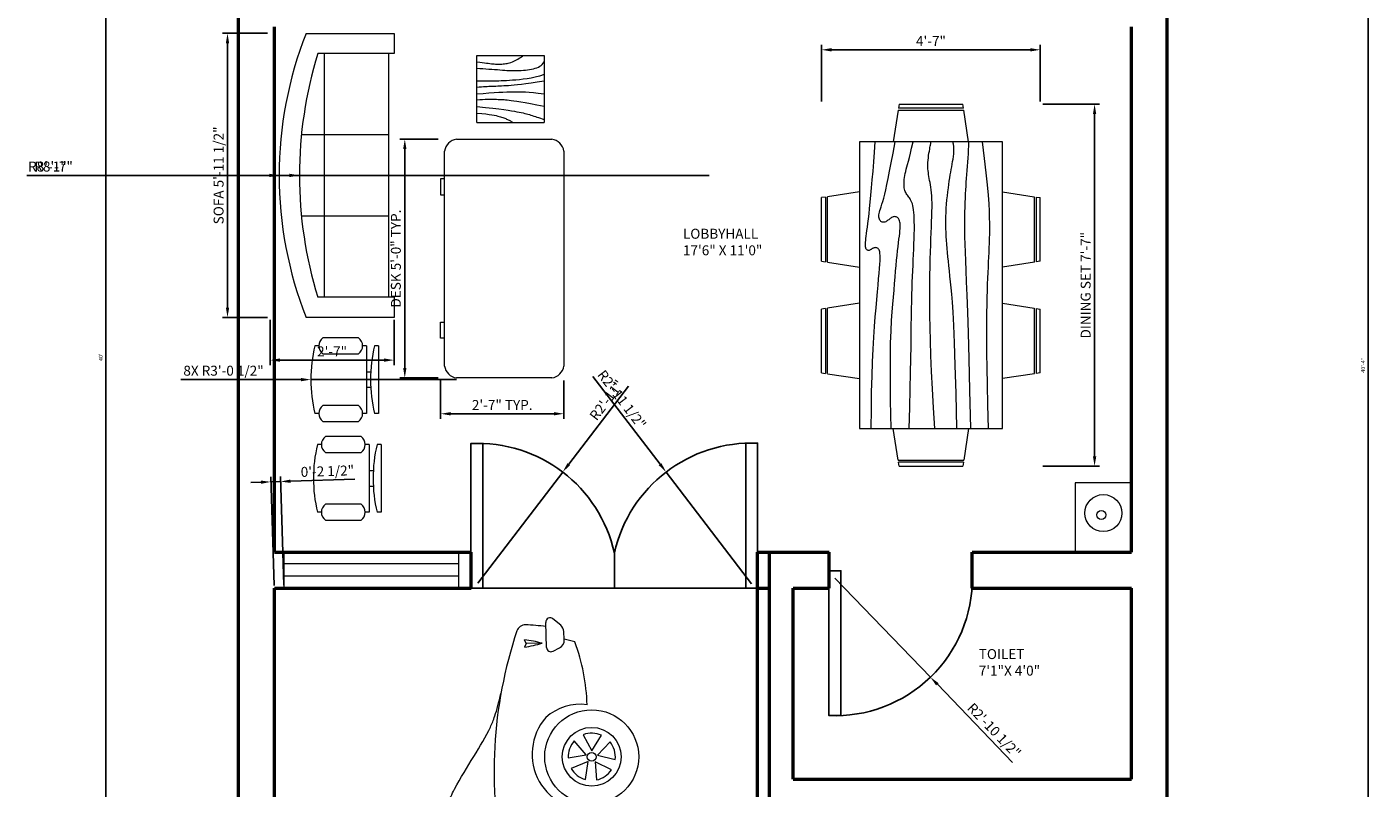
# Model space of a CAD drawing. Units: inches. Extents: x 210 to 950, y 0 to 561.
# Tile 2 of 5: x 210 to 548, y 190 to 382. Entities that reach past the tile are written whole.
import ezdxf

# ---------------------------------------------------------------- set-up
doc = ezdxf.new("R2010")
doc.units = ezdxf.units.IN
for name, color, linetype, lineweight in [('A-ANNO-DIMS', 2, 'Continuous', 18), ('A-AREA-IDEN', 7, 'Continuous', 18), ('A-DOOR', 4, 'Continuous', 25), ('A-FLOR-FIXT', 9, 'Continuous', 18), ('A-FURN', 8, 'Continuous', 18), ('A-GLAZ', 4, 'Continuous', 20), ('A-SITE-VEHI', 8, 'Continuous', 13), ('A-WALL', 7, 'Continuous', 50)]:
    doc.layers.add(name, color=color, linetype=linetype, lineweight=lineweight)
doc.styles.get("Standard").update_dxf_attribs({"font": 'arial.ttf'})
doc.dimstyles.new('ISO-25', dxfattribs={"dimtxt": 2.5, "dimasz": 2.5, "dimexe": 1.25, "dimexo": 0.625, "dimtad": 1, "dimtxsty": 'Standard', "dimcen": 2.5, "dimadec": 0, "dimazin": 0, "dimtfac": 1, "dimtmove": 0, "dimatfit": 3, "dimfxl": 1, "dimarcsym": 0})

# ---------------------------------------------------------------- blocks, each defined once
blk = doc.blocks.new('*U2')
for p, q in [((72.93, 40.23), (85.8, 53.18)), ((75, 38.82), (88.08, 51.97)), ((119.39, 51.91), (117.92, 38.32)), ((50.13, 41.06), (34.31, 40.98)), ((43.26, 39.85), (35.15, 39.78)), ((35.3, 40.46), (50.13, 40.62)), ((111.09, 34.73), (118.48, 34.64)), ((46.65, 26.83), (136.29, 26.77)), ((179.3, 24.35), (180.25, 22.49)), ((180.37, 26.17), (187.51, 26.41)), ((186.68, 22.17), (188.51, 24.37)), ((7.45, 19.78), (9.74, 19.8)), ((10.37, 19.19), (10.38, 18.56)), ((182.62, 21.14), (184.91, 21.28)), ((9.76, 17.93), (8.53, 17.92)), ((50.87, 13.52), (50.91, 10.52))]:
    blk.add_line(p, q)
for points in [[(35.31, 39.93), (35.3, 40.27, 0.269532), (35.14, 40.54), (34.38, 40.96, 0.575383), (34.15, 40.83), (34.15, 40.49, 0.269532), (34.32, 40.22), (35.08, 39.79, 0.575383)], [(28.49, 15.1), (33.61, 14.4), (31.65, 19.18, 0.199906)], [(34.64, 20.05), (35.56, 14.97), (39.5, 18.31, 0.199906)], [(142.85, 15.1), (147.96, 14.4), (146.01, 19.18, 0.199906)], [(148.99, 20.05), (149.91, 14.97), (153.85, 18.31, 0.199906)], [(41.25, 15.74), (36.7, 13.3), (41.09, 10.58, 0.199906)], [(155.6, 15.74), (151.06, 13.3), (155.45, 10.58, 0.199906)], [(31.31, 7.72), (33.55, 12.37), (28.4, 11.99, 0.199906)], [(39.19, 8.12), (35.46, 11.69), (34.23, 6.67, 0.199906)], [(145.66, 7.72), (147.9, 12.37), (142.75, 11.99, 0.199906)], [(153.54, 8.12), (149.81, 11.69), (148.59, 6.67, 0.199906)]]:
    blk.add_lwpolyline(points, format="xyb", close=True)
for points in [[(181.58, 27.46), (181.53, 31.95), (180.48, 32.43)], [(181.58, 27.46), (181.53, 31.95), (182.57, 32.45)], [(50.91, 10.52), (134.38, 11.83)]]:
    blk.add_lwpolyline(points)
for centre, radius in [((115.89, 31.01), 0.619), ((34.98, 13.35), 13.35), ((149.33, 13.35), 13.35), ((34.98, 13.35), 8.35), ((149.33, 13.35), 8.35), ((34.98, 13.35), 1.25), ((149.33, 13.35), 1.25)]:
    blk.add_circle(centre, radius)
for centre, radius, start, end in [((114.6, 105.09), 59.37, 237.6103, 240.9785), ((103.45, -95), 147.78, 83.8163, 95.9705), ((95.51, 3.91), 53.61, 43.2748, 63.5665), ((73.29, 50.49), 10.26, 230.424, 268.0085), ((42.18, -111.35), 149.91, 87.8393, 105.8096), ((20.53, -3.15), 43.06, 98.5304, 116.112), ((80.1, -1364.13), 1402.96, 88.42296, 91.3179), ((118.31, 22.51), 51.16, 161.4307, 193.2363), ((145.17, -84.88), 125.99, 71.5283, 102.1242), ((25.66, 24.94), 94.01, 351.8279, 8.1674), ((184.3, 32.25), 2.49, 357.932, 71.5283), ((79.16, 30.11), 76.3, 177.5773, 185.5205), ((45.64, 26.83), 78.76, 0.852, 4.6556), ((47.43, 26.85), 78.76, 0.852, 4.6556), ((49.23, 26.87), 78.76, 0.852, 4.6556), ((216.26, 37.76), 36.17, 188.4683, 196.5315), ((146.68, 36.98), 36.17, 344.7432, 352.8063), ((116.55, 34.7), 70.29, 353.1942, 357.932), ((34.98, 13.35), 15.9, 0.6373, 176.3412), ((150.1, 14.36), 15.92, 49.2263, 189.1528), ((45.64, 26.83), 78.76, 355.2644, 358.8633), ((47.43, 26.85), 78.76, 355.2644, 358.8633), ((49.23, 26.87), 78.76, 355.2644, 358.8633), ((149.4, 16.55), 14.84, 352.7285, 41.6613), ((180.41, 24.92), 1.25, 91.939, 207.109), ((187.55, 25.16), 1.25, 320.1683, 91.939), ((9.75, 19.18), 0.623, 0.6373, 90.6373), ((182.47, 23.63), 2.49, 207.109, 273.4677), ((114.25, 37.03), 70.29, 344.3985, 346.9385), ((184.76, 23.76), 2.49, 273.4677, 320.1683), ((9.76, 18.55), 0.623, 270.6373, 0.6373), ((162.47, 70.82), 56.18, 271.6865, 290.2774)]:
    blk.add_arc(centre, radius, start, end)
blk.add_ellipse((116.89, 33.59), major_axis=(-0.63, -0.007), ratio=0.610043)
for points, knots in [([(11.39, 38.92), (18.06, 40.19), (30.91, 42.01), (64.77, 40.11), (70.25, 44.91), (82.35, 56.38), (99.18, 57.3), (116.06, 56.35), (133.04, 55.87), (145.24, 49.87), (153.62, 43.8), (161.17, 40.68), (164.92, 39.73), (167.29, 39.15)], [18.629823, 18.629823, 18.629823, 18.629823, 19.527405, 20.700571, 21.107983, 21.608568, 21.92336, 23.151359, 23.716171, 23.908743, 24.77794, 24.943072, 25.187755, 25.187755, 25.187755, 25.187755]), ([(19.11, 14.36), (18.99, 14.21), (18.5, 13.81), (15.35, 15), (9.19, 13.94), (7.26, 22.22), (3.01, 22.66), (1.32, 23.61), (0.64, 26.92), (-0.96, 31.49), (1.54, 32.64), (1.5, 34.06), (1.49, 34.8), (1.49, 35.06), (1.52, 35.3), (1.58, 35.51)], [16.815853, 16.815853, 16.815853, 16.815853, 16.838212, 16.885395, 17.18439, 17.479846, 17.654423, 17.670693, 17.696923, 18.016358, 18.052739, 18.140805, 18.140805, 18.140805, 18.172382, 18.172382, 18.172382, 18.172382])]:
    blk.add_open_spline(points, degree=3, knots=knots)
blk = doc.blocks.new('Sofa - Roundback 7 ft.')
for p, q in [((-12.00002, -32.4421), (-12.00003, -6.5971)), ((11.99997, -32.4421), (11.99998, -6.5971)), ((-36.000027, -34), (-36.000027, -11.4696)), ((35.99998, -34), (35.99998, -11.4696)), ((-35.999844, -13.3819), (35.9998, -13.3819)), ((-36.000027, -32.4421), (35.99998, -32.4421))]:
    blk.add_line(p, q)
for points in [[(-36.000027, -34), (-42.000027, -34), (-42.000027, -8)], [(41.99998, -8), (41.99998, -34), (35.99998, -34)]]:
    blk.add_lwpolyline(points)
for centre, radius, start, end in [((0, -114.25), 114.25, 68.43141, 111.5686), ((-0.00001, -127.1968), 121.1968, 72.72033, 107.2797)]:
    blk.add_arc(centre, radius, start, end)
blk = doc.blocks.new('Chair - Desk')
for p, q in [((-8.5, 0), (-8.5, -1)), ((-8.5, 0), (8.5, 0)), ((8.5, 0), (8.5, -1)), ((-8.5, -3), (-8.5, -4)), ((-8.5, -3), (8.5, -3)), ((-2, -3), (-2, -1.9355)), ((2, -1.9576), (2, -3)), ((8.5, -3), (8.5, -4)), ((-10.5, -5), (-10.5, -14)), ((-6.5, -14), (-6.5, -5)), ((6.5, -5), (6.5, -14)), ((10.5, -14), (10.5, -5)), ((-8.5, -15), (-8.5, -16)), ((8.5, -15), (8.5, -16))]:
    blk.add_line(p, q)
for centre, radius, start, end in [((0, 34.625), 36.625, 256.5803, 283.4197), ((-8.5, -6.5), 2.5, 36.8699, 143.1301), ((8.5, -6.5), 2.5, 36.8699, 143.1301), ((-8.5, -12.5), 2.5, 216.8699, 323.1301), ((0, 19.625), 36.625, 256.5803, 283.4197), ((8.5, -12.5), 2.5, 216.8699, 323.1301)]:
    blk.add_arc(centre, radius, start, end)
blk = doc.blocks.new('Dining Set - 36 x 72 in.')
for p, q in [((-22, 27.5), (-22.1562, 26.50042)), ((-22, 27.5), (-6, 27.5)), ((-5.8437, 26.49966), (-6, 27.5)), ((6, 27.5), (5.8438, 26.50042)), ((6, 27.5), (22, 27.5)), ((22.1563, 26.49966), (22, 27.5)), ((-22.2343, 26.00059), (-23.4847, 17.99762)), ((-22.2304, 26), (-5.7608, 26)), ((-5.8416, 26.5), (-22.1534, 26.5)), ((-4.5152, 17.99762), (-5.7655, 25.99926)), ((5.7657, 26.00059), (4.5153, 17.99762)), ((5.7696, 26), (22.2392, 26)), ((22.1584, 26.5), (5.8466, 26.5)), ((23.4848, 17.99762), (22.2345, 25.99926)), ((36, 18), (-36, 18)), ((-36, 18), (-36, -18)), ((36, -18), (36, 18)), ((-45.5, 8), (-44.5004, 8.15617)), ((-45.5, 8), (-45.5, -8)), ((-44.5, -8.15843), (-44.5, 8.15338)), ((-44.0006, 8.23428), (-35.9976, 9.48474)), ((-44, 8.23041), (-44, -8.23915)), ((44.0006, 8.23428), (35.9976, 9.48474)), ((44, 8.23041), (44, -8.23915)), ((44.5, -8.15843), (44.5, 8.15338)), ((45.5, 8), (44.5005, 8.15617)), ((45.5, 8), (45.5, -8)), ((-44.4997, -8.15631), (-45.5, -8)), ((-35.9976, -9.48476), (-43.9993, -8.2345)), ((35.9976, -9.48476), (43.9993, -8.2345)), ((44.4997, -8.15631), (45.5, -8)), ((-36, -18), (36, -18)), ((-22.2343, -26.0006), (-23.4847, -17.99762)), ((-4.5152, -17.99762), (-5.7655, -25.99928)), ((5.7657, -26.0006), (4.5153, -17.99762)), ((23.4848, -17.99762), (22.2345, -25.99928)), ((-22.2304, -26), (-5.7608, -26)), ((-22, -27.5), (-22.1562, -26.50044)), ((-5.8416, -26.5), (-22.1534, -26.5)), ((-5.8437, -26.49967), (-6, -27.5)), ((5.7696, -26), (22.2392, -26)), ((6, -27.5), (5.8438, -26.50044)), ((22.1584, -26.5), (5.8466, -26.5)), ((22.1563, -26.49967), (22, -27.5)), ((-22, -27.5), (-6, -27.5)), ((6, -27.5), (22, -27.5))]:
    blk.add_line(p, q)
for points in [[(-36, 15), (-31.1772, 14.97754), (-26.8079, 14.91406), (-22.8538, 14.81543), (-19.276, 14.6875), (-16.0362, 14.53613), (-13.0957, 14.36718), (-10.4159, 14.18652), (-7.9583, 14), (-5.6904, 13.81315), (-3.6035, 13.63021), (-1.6954, 13.45508), (0.0365, 13.29166), (1.5945, 13.14388), (2.9811, 13.01562), (4.1988, 12.9108), (5.25, 12.83333), (6.1393, 12.78613), (6.8802, 12.76823), (7.4883, 12.77767), (7.9792, 12.8125), (8.3685, 12.87077), (8.6719, 12.95052), (8.9049, 13.0498), (9.0833, 13.16666), (9.2205, 13.29899), (9.3216, 13.44401), (9.3895, 13.59879), (9.4271, 13.76041), (9.4373, 13.92594), (9.4232, 14.09245), (9.3875, 14.257), (9.3333, 14.41666), (9.2638, 14.56917), (9.1836, 14.71484), (9.0975, 14.85465), (9.0104, 14.98958), (8.9272, 15.1206), (8.8529, 15.2487), (8.7922, 15.37483), (8.75, 15.5), (8.7305, 15.62467), (8.7344, 15.74739), (8.7617, 15.86621), (8.8125, 15.97916), (8.8867, 16.08431), (8.9844, 16.17968), (9.1055, 16.26334), (9.25, 16.33333), (9.4189, 16.38802), (9.6172, 16.42708), (9.8506, 16.45052), (10.125, 16.45833), (10.4463, 16.45052), (10.8203, 16.42708), (11.2529, 16.38802), (11.75, 16.33333), (12.3184, 16.26318), (12.9694, 16.17838), (13.7151, 16.07991), (14.5677, 15.96875), (15.5395, 15.84586), (16.6426, 15.71224), (17.8893, 15.56884), (19.2917, 15.41666), (20.859, 15.25667), (22.5879, 15.08984), (24.4721, 14.91715), (26.5052, 14.73958), (28.6809, 14.5581), (30.9929, 14.3737), (33.4347, 14.18733), (36, 14)], [(-36, 10), (-28.9766, 10.14274), (-23.1725, 10.20442), (-18.4241, 10.19775), (-14.5677, 10.13541), (-11.4399, 10.03011), (-8.877, 9.89453), (-6.7154, 9.74137), (-4.7917, 9.58333), (-2.9698, 9.43082), (-1.2246, 9.28515), (0.4415, 9.14534), (2.026, 9.01041), (3.5266, 8.87939), (4.9408, 8.7513), (6.266, 8.62516), (7.5, 8.5), (8.6411, 8.37549), (9.6914, 8.2539), (10.6538, 8.13818), (11.5312, 8.03125), (12.3267, 7.93603), (13.043, 7.85547), (13.6831, 7.79248), (14.25, 7.75), (14.7471, 7.7303), (15.1797, 7.73307), (15.5537, 7.75732), (15.875, 7.80208), (16.1494, 7.86637), (16.3828, 7.94922), (16.5811, 8.04964), (16.75, 8.16666), (16.8944, 8.29915), (17.0143, 8.44531), (17.1089, 8.60319), (17.1771, 8.77083), (17.218, 8.94629), (17.2305, 9.1276), (17.2137, 9.31282), (17.1667, 9.5), (17.0895, 9.6875), (16.987, 9.875), (16.8649, 10.0625), (16.7292, 10.25), (16.5856, 10.4375), (16.4401, 10.625), (16.2985, 10.8125), (16.1667, 11), (16.05, 11.18733), (15.9518, 11.3737), (15.8752, 11.5581), (15.8229, 11.73958), (15.798, 11.91715), (15.8034, 12.08984), (15.842, 12.25667), (15.9167, 12.41666), (16.0295, 12.56836), (16.1784, 12.70833), (16.3605, 12.83268), (16.5729, 12.9375), (16.8127, 13.01888), (17.0768, 13.07291), (17.3625, 13.0957), (17.6667, 13.08333), (17.9894, 13.03312), (18.3418, 12.94726), (18.7382, 12.82918), (19.1927, 12.68229), (19.7195, 12.51001), (20.3327, 12.31575), (21.0465, 12.10294), (21.875, 11.875), (22.8357, 11.63354), (23.959, 11.37304), (25.2786, 11.08618), (26.8282, 10.76562), (28.6414, 10.40405), (30.752, 9.99414), (33.1936, 9.52856), (36, 9)], [(-36, 5.5), (-30.7157, 5.3348), (-26.069, 5.20963), (-21.9946, 5.11767), (-18.4271, 5.05208), (-15.3009, 5.00602), (-12.5508, 4.97265), (-10.1112, 4.94515), (-7.9167, 4.91666), (-5.909, 4.88167), (-4.0586, 4.83984), (-2.3429, 4.79215), (-0.7396, 4.73958), (0.7739, 4.6831), (2.22, 4.6237), (3.6213, 4.56233), (5, 4.5), (6.373, 4.43782), (7.7344, 4.3776), (9.0723, 4.32129), (10.375, 4.27083), (11.6309, 4.22819), (12.8281, 4.19531), (13.9551, 4.17415), (15, 4.16666), (15.954, 4.17448), (16.819, 4.19791), (17.6001, 4.23698), (18.3021, 4.29166), (18.9299, 4.36198), (19.4883, 4.44791), (19.9823, 4.54948), (20.4167, 4.66666), (20.7969, 4.79899), (21.1302, 4.94401), (21.4245, 5.09879), (21.6875, 5.26041), (21.9271, 5.42594), (22.1511, 5.59245), (22.3672, 5.757), (22.5834, 5.91666), (22.8065, 6.06868), (23.0404, 6.21093), (23.2879, 6.34147), (23.5521, 6.45833), (23.8358, 6.55957), (24.142, 6.64323), (24.4735, 6.70735), (24.8334, 6.75), (25.2235, 6.76969), (25.642, 6.76692), (26.0858, 6.74267), (26.5521, 6.69791), (27.0379, 6.63362), (27.5404, 6.55078), (28.0565, 6.45036), (28.5834, 6.33333), (29.1242, 6.19987), (29.7071, 6.04687), (30.3661, 5.87044), (31.1354, 5.66666), (32.0493, 5.43164), (33.142, 5.16146), (34.4475, 4.85221), (36, 4.5)], [(-36, -1), (-30.7915, -0.6591), (-26.0195, -0.38216), (-21.6519, -0.16284), (-17.6563, 0.00521), (-14.0005, 0.12833), (-10.6523, 0.21289), (-7.5796, 0.26522), (-4.75, 0.29166), (-2.134, 0.29793), (0.2878, 0.28711), (2.5317, 0.26163), (4.6146, 0.22396), (6.5529, 0.17651), (8.3633, 0.12174), (10.0623, 0.06209), (11.6667, 0), (13.1899, -0.06201), (14.6341, -0.1211), (15.9982, -0.17432), (17.2813, -0.21875), (18.4823, -0.25147), (19.6003, -0.26953), (20.6343, -0.27002), (21.5834, -0.25), (22.4481, -0.20768), (23.2357, -0.14584), (23.9549, -0.06836), (24.6146, 0.02083), (25.2235, 0.11784), (25.7904, 0.21875), (26.3241, 0.31966), (26.8334, 0.41666), (27.3265, 0.50618), (27.8099, 0.58593), (28.2894, 0.65397), (28.7709, 0.70833), (29.2601, 0.74707), (29.763, 0.76823), (30.2855, 0.76985), (30.8334, 0.75), (31.4088, 0.70784), (31.9994, 0.64713), (32.589, 0.57275), (33.1615, 0.48958), (33.7008, 0.4025), (34.1908, 0.3164), (34.6153, 0.23616), (34.9584, 0.16666), (35.2099, 0.11165), (35.3848, 0.07031), (35.504, 0.04069), (35.5886, 0.02083), (35.6594, 0.00879), (35.7377, 0.0026), (35.8442, 0.00032), (36, 0)], [(-36, -6.5), (-27.1843, -6.31267), (-20.084, -6.1263), (-14.469, -5.9419), (-10.1094, -5.76042), (-6.7752, -5.58285), (-4.2363, -5.41016), (-2.2629, -5.24333), (-0.625, -5.08334), (0.8708, -4.93099), (2.2715, -4.78646), (3.5872, -4.64974), (4.8281, -4.52084), (6.0046, -4.39974), (7.127, -4.28646), (8.2053, -4.18099), (9.25, -4.08334), (10.2705, -3.99382), (11.2734, -3.91407), (12.2647, -3.84603), (13.25, -3.79167), (14.2354, -3.75293), (15.2266, -3.73177), (16.2295, -3.73015), (17.25, -3.75), (18.2912, -3.79248), (19.3451, -3.85547), (20.4009, -3.93604), (21.4479, -4.03125), (22.4754, -4.13819), (23.4727, -4.25391), (24.4289, -4.37549), (25.3334, -4.5), (26.1785, -4.62492), (26.9694, -4.74935), (27.7145, -4.87281), (28.4219, -4.99479), (29.1, -5.11483), (29.7572, -5.23242), (30.4016, -5.34709), (31.0417, -5.45834), (31.6837, -5.56437), (32.3262, -5.65821), (32.9658, -5.73153), (33.599, -5.77604), (34.2224, -5.78345), (34.8327, -5.74545), (35.4264, -5.65373), (36, -5.5)], [(-36, -10), (-26.4022, -9.81299), (-18.4675, -9.62891), (-11.9839, -9.45069), (-6.7396, -9.28125), (-2.5226, -9.12354), (0.8789, -8.98047), (3.6769, -8.85498), (6.0833, -8.75), (8.2767, -8.66765), (10.3021, -8.60677), (12.1712, -8.56543), (13.8958, -8.54167), (15.4876, -8.53353), (16.9583, -8.53907), (18.3197, -8.55632), (19.5834, -8.58334), (20.7616, -8.61841), (21.8685, -8.66081), (22.9188, -8.71004), (23.9271, -8.76563), (24.9081, -8.82707), (25.8763, -8.89388), (26.8465, -8.96558), (27.8334, -9.04167), (28.8474, -9.12118), (29.8828, -9.20117), (30.93, -9.27824), (31.9792, -9.34896), (33.0205, -9.40991), (34.0443, -9.45768), (35.0407, -9.48885), (36, -9.5)], [(-36, -14.5), (-30.0881, -14.33513), (-25.0332, -14.21224), (-20.7312, -14.12647), (-17.0781, -14.07292), (-13.97, -14.04671), (-11.3027, -14.04297), (-8.9724, -14.05681), (-6.875, -14.08334), (-4.9224, -14.11833), (-3.0905, -14.16016), (-1.3709, -14.20785), (0.2448, -14.26042), (1.7647, -14.3169), (3.1973, -14.3763), (4.5507, -14.43767), (5.8333, -14.5), (7.0554, -14.5621), (8.235, -14.62175), (9.3922, -14.67652), (10.5469, -14.72396), (11.7192, -14.76164), (12.929, -14.78711), (14.1965, -14.79794), (15.5417, -14.79167), (16.9933, -14.76424), (18.6152, -14.70508), (20.4804, -14.60197), (22.6615, -14.44271), (25.2312, -14.21509), (28.2624, -13.9069), (31.8277, -13.50594), (36, -13)]]:
    blk.add_lwpolyline(points)
blk = doc.blocks.new('Desk - 30 x 60 in.')
for p, q in [((-26.999995, 0), (26.999995, 0)), ((-29.999995, -27), (-29.999995, -3)), ((29.999995, -3), (29.999995, -27)), ((26.999995, -30), (-26.999995, -30)), ((-20.000005, -30), (-20.000005, -31)), ((-16.000005, -31), (-16.000005, -30)), ((15.999995, -31), (15.999995, -30)), ((19.999995, -30), (19.999995, -31)), ((-20.000005, -31), (-16.000005, -31)), ((19.999995, -31), (15.999995, -31))]:
    blk.add_line(p, q)
for centre, start, end in [((-26.499995, -3.5), 98.1301, 171.8699), ((26.499995, -3.5), 8.130102, 81.8699), ((-26.499995, -26.5), 188.1301, 261.8699), ((26.499995, -26.5), 278.1301, 351.8699)]:
    blk.add_arc(centre, 3.535534, start, end)
blk = doc.blocks.new('Table - Square Woodgrain 42 x 42 in.')
blk.add_line((0, -42), (42, -42))
for points in [[(0, -4), (1.704, -4.2172), (3.2358, -4.4188), (4.615, -4.604), (5.8615, -4.7721), (6.9951, -4.9224), (8.0357, -5.0541), (9.0031, -5.1667), (9.9171, -5.2594), (10.7951, -5.3316), (11.6445, -5.3836), (12.4702, -5.4157), (13.277, -5.4283), (14.0698, -5.4217), (14.8535, -5.3964), (15.6331, -5.3526), (16.4133, -5.2908), (17.1986, -5.2103), (17.9913, -5.1062), (18.793, -4.9727), (19.6056, -4.8038), (20.4307, -4.5937), (21.2701, -4.3365), (22.1256, -4.0262), (22.9989, -3.6571), (23.888, -3.2272), (24.7756, -2.7516), (25.6408, -2.2491), (26.4624, -1.7387), (27.2195, -1.2395), (27.891, -0.7703), (28.456, -0.3501), (28.8934, 0.002)], [(0, -42), (0, 0), (42, 0), (42, -42)], [(0, -8), (1.8203, -8.1001), (3.6741, -8.2149), (5.5411, -8.3408), (7.4011, -8.4741), (9.2339, -8.6112), (11.0193, -8.7484), (12.7371, -8.8821), (14.3671, -9.0086), (15.8954, -9.1246), (17.3337, -9.2278), (18.6997, -9.3159), (20.0116, -9.387), (21.2871, -9.4389), (22.5442, -9.4696), (23.8008, -9.477), (25.0749, -9.459), (26.3791, -9.4137), (27.7049, -9.3403), (29.0383, -9.2382), (30.3655, -9.1068), (31.6728, -8.9455), (32.9461, -8.7535), (34.1717, -8.5304), (35.3358, -8.2756), (36.4268, -7.9863), (37.443, -7.6521), (38.3849, -7.2603), (39.253, -6.7986), (40.048, -6.2542), (40.7705, -5.6147), (41.421, -4.8674), (42, -4)], [(42, -12), (39.1784, -12.8621), (36.4519, -13.5654), (33.8246, -14.1294), (31.3004, -14.5731), (28.8832, -14.9161), (26.577, -15.1775), (24.3858, -15.3768), (22.3136, -15.5332), (20.3622, -15.6632), (18.5254, -15.7718), (16.7947, -15.8612), (15.1618, -15.9338), (13.6183, -15.9916), (12.1558, -16.0369), (10.7659, -16.0718), (9.4403, -16.0987), (8.1703, -16.1191), (6.9461, -16.1325), (5.7577, -16.1377), (4.595, -16.1335), (3.4479, -16.1188), (2.3064, -16.0924), (1.1604, -16.0532), (0, -16)], [(42, -16), (37.6529, -16.7365), (33.8802, -17.329), (30.6179, -17.7961), (27.8015, -18.1561), (25.3668, -18.4275), (23.2497, -18.6288), (21.3859, -18.7785), (19.7111, -18.8949), (18.1693, -18.9939), (16.7375, -19.0795), (15.401, -19.1534), (14.1449, -19.217), (12.9544, -19.2717), (11.8148, -19.3191), (10.7113, -19.3606), (9.6291, -19.3976), (8.5534, -19.4323), (7.47, -19.4689), (6.3643, -19.5122), (5.222, -19.5672), (4.0288, -19.6386), (2.7703, -19.7313), (1.4321, -19.8501), (0, -20)], [(0, -24), (3.9243, -23.6805), (7.4766, -23.4138), (10.6891, -23.1954), (13.5943, -23.0205), (16.2247, -22.8847), (18.6125, -22.7832), (20.7903, -22.7116), (22.7903, -22.6651), (24.6563, -22.642), (26.4764, -22.6507), (28.35, -22.7024), (30.3766, -22.8084), (32.6555, -22.98), (35.2861, -23.2283), (38.3678, -23.5645), (42, -24)], [(42, -32), (37.392, -31.017), (33.4585, -30.2231), (30.1291, -29.5949), (27.3334, -29.109), (25.0009, -28.742), (23.0612, -28.4707), (21.4439, -28.2716), (20.0786, -28.1215), (18.8998, -28.0002), (17.8609, -27.9014), (16.9206, -27.8219), (16.0371, -27.7588), (15.1691, -27.709), (14.2748, -27.6693), (13.3128, -27.6368), (12.2415, -27.6083), (11.0295, -27.5824), (9.6867, -27.5643), (8.233, -27.5608), (6.6884, -27.5787), (5.0728, -27.6248), (3.4062, -27.7058), (1.7086, -27.8286), (0, -28)], [(0, -32), (5.4026, -32.5358), (9.9494, -33.019), (13.7424, -33.4553), (16.8834, -33.8505), (19.4743, -34.2106), (21.6171, -34.5413), (23.4136, -34.8486), (24.9657, -35.1382), (26.3614, -35.4156), (27.6332, -35.6841), (28.7995, -35.9467), (29.8788, -36.2064), (30.8897, -36.4661), (31.8507, -36.7288), (32.7802, -36.9973), (33.6968, -37.2747), (34.6175, -37.5635), (35.5531, -37.8651), (36.5128, -38.1805), (37.506, -38.5108), (38.5421, -38.8568), (39.6302, -39.2197), (40.7797, -39.6004), (42, -40)], [(0, -36), (3.0098, -36.2857), (5.5354, -36.5643), (7.6368, -36.8359), (9.374, -37.1009), (10.807, -37.3597), (11.9957, -37.6126), (13.0002, -37.8599), (13.8804, -38.102), (14.6874, -38.3393), (15.4365, -38.5729), (16.1338, -38.8041), (16.7858, -39.0341), (17.3987, -39.264), (17.9787, -39.4952), (18.5322, -39.7288), (19.0655, -39.9662), (19.5832, -40.2081), (20.0842, -40.4544), (20.5657, -40.7046), (21.0249, -40.9581), (21.459, -41.2144), (21.8653, -41.4731), (22.2409, -41.7335), (22.5831, -41.9951)]]:
    blk.add_lwpolyline(points)
blk = doc.blocks.new('*D15')
at = {"layer": 'A-ANNO-DIMS', "color": 0, "lineweight": -2, "transparency": 16777216}
for p, q in [((262.29, 538.5), (228.3, 538.5)), ((229.55, 61), (229.55, 536)), ((262.29, 58.5), (228.3, 58.5))]:
    blk.add_line(p, q, dxfattribs=at)
at = {"layer": 'A-ANNO-DIMS', "color": 0, "transparency": 16777216}
for points in [[(229.13, 536), (229.96, 536), (229.55, 538.5)], [(229.13, 61), (229.96, 61), (229.55, 58.5)]]:
    blk.add_solid(points, dxfattribs=at)
at = {"layer": 'Defpoints', "color": 0, "transparency": 16777216}
for p in [(229.55, 538.5), (262.91, 538.5), (262.91, 58.5)]:
    blk.add_point(p, dxfattribs=at)
at = {"layer": 'A-ANNO-DIMS', "color": 0, "transparency": 16777216, "insert": (228.41, 298.5), "char_height": 1, "attachment_point": 5, "rotation": 90}
blk.add_mtext("40'", dxfattribs=at)
blk = doc.blocks.new('*D16')
at = {"layer": 'A-ANNO-DIMS', "color": 0, "lineweight": -2, "transparency": 16777216}
for p, q in [((497.04, 538.5), (548.19, 538.5)), ((546.94, 57), (546.94, 536)), ((497.04, 54.5), (548.19, 54.5))]:
    blk.add_line(p, q, dxfattribs=at)
at = {"layer": 'A-ANNO-DIMS', "color": 0, "transparency": 16777216}
for points in [[(546.52, 536), (547.35, 536), (546.94, 538.5)], [(546.52, 57), (547.35, 57), (546.94, 54.5)]]:
    blk.add_solid(points, dxfattribs=at)
at = {"layer": 'Defpoints', "color": 0, "transparency": 16777216}
for p in [(496.41, 538.5), (546.94, 538.5), (496.41, 54.5)]:
    blk.add_point(p, dxfattribs=at)
at = {"layer": 'A-ANNO-DIMS', "color": 0, "transparency": 16777216, "insert": (545.8, 296.5), "char_height": 1, "attachment_point": 5, "rotation": 90}
blk.add_mtext('40\'-4"', dxfattribs=at)
blk = doc.blocks.new('WIN-44IN-DEEP-FRAME')
for p, q in [((0, 0), (0, 9)), ((0, 9), (43.89, 9)), ((43.89, 9), (43.89, 0)), ((43.89, 6), (0, 6)), ((0, 3), (43.89, 3)), ((43.89, 0), (0, 0))]:
    blk.add_line(p, q)
blk = doc.blocks.new('DOOR-LEAF-36IN')
blk.add_lwpolyline([(0, 0), (0, -2.99), (-36.41, -2.99), (-36.41, 0)], close=True)
blk = doc.blocks.new('*D42')
at = {"layer": 'A-ANNO-DIMS', "color": 0, "lineweight": -2, "transparency": 16777216}
for p, q in [((270.22, 379.9), (258.88, 379.9)), ((260.13, 310.99), (260.13, 377.4)), ((270.22, 308.49), (258.88, 308.49))]:
    blk.add_line(p, q, dxfattribs=at)
at = {"layer": 'A-ANNO-DIMS', "color": 0, "transparency": 16777216}
for points in [[(259.72, 377.4), (260.55, 377.4), (260.13, 379.9)], [(259.72, 310.99), (260.55, 310.99), (260.13, 308.49)]]:
    blk.add_solid(points, dxfattribs=at)
at = {"layer": 'Defpoints', "color": 0, "transparency": 16777216}
for p in [(260.13, 379.9), (270.84, 379.9), (270.84, 308.49)]:
    blk.add_point(p, dxfattribs=at)
at = {"layer": 'A-ANNO-DIMS', "color": 0, "transparency": 16777216, "insert": (258.22, 344.2), "char_height": 2.5, "attachment_point": 5, "rotation": 90}
blk.add_mtext('SOFA 5\'-11 1/2"', dxfattribs=at)
blk = doc.blocks.new('*D43')
at = {"layer": 'A-ANNO-DIMS', "color": 0, "lineweight": -2, "transparency": 16777216}
for p, q in [((270.84, 307.87), (270.84, 296.53)), ((302.01, 307.87), (302.01, 296.53)), ((299.51, 297.78), (273.34, 297.78))]:
    blk.add_line(p, q, dxfattribs=at)
at = {"layer": 'A-ANNO-DIMS', "color": 0, "transparency": 16777216}
for points in [[(273.34, 298.2), (273.34, 297.37), (270.84, 297.78)], [(299.51, 298.2), (299.51, 297.37), (302.01, 297.78)]]:
    blk.add_solid(points, dxfattribs=at)
at = {"layer": 'Defpoints', "color": 0, "transparency": 16777216}
for p in [(270.84, 308.49), (302.01, 308.49), (270.84, 297.78)]:
    blk.add_point(p, dxfattribs=at)
at = {"layer": 'A-ANNO-DIMS', "color": 0, "transparency": 16777216, "insert": (286.43, 299.66), "char_height": 2.5, "attachment_point": 5}
blk.add_mtext('2\'-7"', dxfattribs=at)
blk = doc.blocks.new('*D44')
at = {"layer": 'A-ANNO-DIMS', "color": 0, "lineweight": -2, "transparency": 16777216}
for p, q in [((313.09, 353.3), (303.46, 353.3)), ((304.71, 350.8), (304.71, 295.8)), ((313.09, 293.3), (303.46, 293.3))]:
    blk.add_line(p, q, dxfattribs=at)
at = {"layer": 'A-ANNO-DIMS', "color": 0, "transparency": 16777216}
for points in [[(304.3, 350.8), (305.13, 350.8), (304.71, 353.3)], [(304.3, 295.8), (305.13, 295.8), (304.71, 293.3)]]:
    blk.add_solid(points, dxfattribs=at)
at = {"layer": 'Defpoints', "color": 0, "transparency": 16777216}
for p in [(313.71, 353.3), (304.71, 293.3), (313.71, 293.3)]:
    blk.add_point(p, dxfattribs=at)
at = {"layer": 'A-ANNO-DIMS', "color": 0, "transparency": 16777216, "insert": (302.79, 323.3), "char_height": 2.5, "attachment_point": 5, "rotation": 90}
blk.add_mtext('DESK 5\'-0" TYP.', dxfattribs=at)
blk = doc.blocks.new('*D45')
at = {"layer": 'A-ANNO-DIMS', "color": 0, "lineweight": -2, "transparency": 16777216}
for p, q in [((313.71, 292.68), (313.71, 283.05)), ((344.71, 292.68), (344.71, 283.05)), ((316.21, 284.3), (342.21, 284.3))]:
    blk.add_line(p, q, dxfattribs=at)
at = {"layer": 'A-ANNO-DIMS', "color": 0, "transparency": 16777216}
for points in [[(316.21, 284.72), (316.21, 283.89), (313.71, 284.3)], [(342.21, 284.72), (342.21, 283.89), (344.71, 284.3)]]:
    blk.add_solid(points, dxfattribs=at)
at = {"layer": 'Defpoints', "color": 0, "transparency": 16777216}
for p in [(313.71, 293.3), (344.71, 293.3), (344.71, 284.3)]:
    blk.add_point(p, dxfattribs=at)
at = {"layer": 'A-ANNO-DIMS', "color": 0, "transparency": 16777216, "insert": (329.21, 286.19), "char_height": 2.5, "attachment_point": 5}
blk.add_mtext('2\'-7" TYP.', dxfattribs=at)
blk = doc.blocks.new('*D46')
at = {"layer": 'A-ANNO-DIMS', "color": 0, "lineweight": -2, "transparency": 16777216}
for p, q in [((465.13, 362.11), (479.41, 362.11)), ((478.16, 273.61), (478.16, 359.61)), ((465.13, 271.11), (479.41, 271.11))]:
    blk.add_line(p, q, dxfattribs=at)
at = {"layer": 'A-ANNO-DIMS', "color": 0, "transparency": 16777216}
for points in [[(477.74, 359.61), (478.58, 359.61), (478.16, 362.11)], [(477.74, 273.61), (478.58, 273.61), (478.16, 271.11)]]:
    blk.add_solid(points, dxfattribs=at)
at = {"layer": 'Defpoints', "color": 0, "transparency": 16777216}
for p in [(464.51, 362.11), (478.16, 362.11), (464.51, 271.11)]:
    blk.add_point(p, dxfattribs=at)
at = {"layer": 'A-ANNO-DIMS', "color": 0, "transparency": 16777216, "insert": (476.24, 316.61), "char_height": 2.5, "attachment_point": 5, "rotation": 90}
blk.add_mtext('DINING SET 7\'-7"', dxfattribs=at)
blk = doc.blocks.new('*D47')
at = {"layer": 'A-ANNO-DIMS', "color": 0, "lineweight": -2, "transparency": 16777216}
for p, q in [((409.51, 362.73), (409.51, 377.01)), ((462.01, 375.76), (412.01, 375.76)), ((464.51, 362.73), (464.51, 377.01))]:
    blk.add_line(p, q, dxfattribs=at)
at = {"layer": 'A-ANNO-DIMS', "color": 0, "transparency": 16777216}
for points in [[(412.01, 376.17), (412.01, 375.34), (409.51, 375.76)], [(462.01, 376.17), (462.01, 375.34), (464.51, 375.76)]]:
    blk.add_solid(points, dxfattribs=at)
at = {"layer": 'Defpoints', "color": 0, "transparency": 16777216}
for p in [(409.51, 375.76), (409.51, 362.11), (464.51, 362.11)]:
    blk.add_point(p, dxfattribs=at)
at = {"layer": 'A-ANNO-DIMS', "color": 0, "transparency": 16777216, "insert": (437.01, 377.63), "char_height": 2.5, "attachment_point": 5}
blk.add_mtext('4\'-7"', dxfattribs=at)
blk = doc.blocks.new('*D52')
at = {"layer": 'A-ANNO-DIMS', "color": 0, "lineweight": -2, "transparency": 16777216}
for p, q in [((271.89, 241.13), (270.99, 268.44)), ((274.32, 241.21), (273.43, 268.52)), ((275.96, 267.35), (292.18, 267.88)), ((268.54, 267.11), (266.04, 267.02)), ((271.03, 267.19), (273.47, 267.27))]:
    blk.add_line(p, q, dxfattribs=at)
at = {"layer": 'A-ANNO-DIMS', "color": 0, "transparency": 16777216}
for points in [[(268.52, 267.52), (268.55, 266.69), (271.03, 267.19)], [(275.95, 267.77), (275.98, 266.93), (273.47, 267.27)]]:
    blk.add_solid(points, dxfattribs=at)
at = {"layer": 'Defpoints', "color": 0, "transparency": 16777216}
for p in [(273.47, 267.27), (271.91, 240.5), (274.34, 240.58)]:
    blk.add_point(p, dxfattribs=at)
at = {"layer": 'A-ANNO-DIMS', "color": 0, "transparency": 16777216, "insert": (285.26, 269.57), "char_height": 2.5, "attachment_point": 5, "rotation": 1.8816}
blk.add_mtext('0\'-2 1/2"', dxfattribs=at)
blk = doc.blocks.new('*D55')
at = {"layer": 'A-ANNO-DIMS', "color": 0, "lineweight": -2, "transparency": 16777216}
for p, q in [((352.03, 293.7), (368.9, 271.65)), ((391.93, 241.55), (370.42, 269.66))]:
    blk.add_line(p, q, dxfattribs=at)
at = {"layer": 'A-ANNO-DIMS', "color": 0, "transparency": 16777216}
blk.add_solid([(369.23, 271.9), (368.57, 271.39), (370.42, 269.66)], dxfattribs=at)
at = {"layer": 'Defpoints', "color": 0, "transparency": 16777216}
for p in [(370.42, 269.66), (391.93, 241.55)]:
    blk.add_point(p, dxfattribs=at)
at = {"layer": 'A-ANNO-DIMS', "color": 0, "transparency": 16777216, "insert": (359.04, 287.69), "char_height": 2.5, "attachment_point": 5, "rotation": 307.4181}
blk.add_mtext('R2\'-11 1/2"', dxfattribs=at)
blk = doc.blocks.new('*D56')
at = {"layer": 'A-ANNO-DIMS', "color": 0, "lineweight": -2, "transparency": 16777216}
for p, q in [((360.94, 291.26), (345.94, 271.64)), ((323.09, 241.73), (344.42, 269.65))]:
    blk.add_line(p, q, dxfattribs=at)
at = {"layer": 'A-ANNO-DIMS', "color": 0, "transparency": 16777216}
blk.add_solid([(345.61, 271.89), (346.27, 271.38), (344.42, 269.65)], dxfattribs=at)
at = {"layer": 'Defpoints', "color": 0, "transparency": 16777216}
for p in [(344.42, 269.65), (323.09, 241.73)]:
    blk.add_point(p, dxfattribs=at)
at = {"layer": 'A-ANNO-DIMS', "color": 0, "transparency": 16777216, "insert": (355.73, 287.54), "char_height": 2.5, "attachment_point": 5, "rotation": 52.6128}
blk.add_mtext('R2\'-11"', dxfattribs=at)
blk = doc.blocks.new('*D57')
at = {"layer": 'A-ANNO-DIMS', "color": 0, "lineweight": -2, "transparency": 16777216}
for p, q in [((412.87, 242.99), (436.88, 218.12)), ((457.56, 196.7), (438.62, 216.32))]:
    blk.add_line(p, q, dxfattribs=at)
at = {"layer": 'A-ANNO-DIMS', "color": 0, "transparency": 16777216}
blk.add_solid([(438.92, 216.61), (438.32, 216.03), (436.88, 218.12)], dxfattribs=at)
at = {"layer": 'Defpoints', "color": 0, "transparency": 16777216}
for p in [(412.87, 242.99), (436.88, 218.12)]:
    blk.add_point(p, dxfattribs=at)
at = {"layer": 'A-ANNO-DIMS', "color": 0, "transparency": 16777216, "insert": (452.67, 204.53), "char_height": 2.5, "attachment_point": 5, "rotation": 313.9912}
blk.add_mtext('R2\'-10 1/2"', dxfattribs=at)
blk = doc.blocks.new('*D65')
at = {"layer": 'A-ANNO-DIMS', "color": 0, "lineweight": -2, "transparency": 16777216}
for p, q in [((211.25, 344.19), (275.71, 344.19)), ((381.23, 344.19), (278.21, 344.19))]:
    blk.add_line(p, q, dxfattribs=at)
at = {"layer": 'A-ANNO-DIMS', "color": 0, "transparency": 16777216}
blk.add_solid([(275.71, 344.61), (275.71, 343.78), (278.21, 344.19)], dxfattribs=at)
at = {"layer": 'Defpoints', "color": 0, "transparency": 16777216}
for p in [(278.21, 344.19), (381.23, 344.19)]:
    blk.add_point(p, dxfattribs=at)
at = {"layer": 'A-ANNO-DIMS', "color": 0, "transparency": 16777216, "insert": (216.4, 346.1), "char_height": 2.5, "attachment_point": 5}
blk.add_mtext('R8\'-7"', dxfattribs=at)
blk = doc.blocks.new('*D66')
at = {"layer": 'A-ANNO-DIMS', "color": 0, "lineweight": -2, "transparency": 16777216}
for p, q in [((209.7, 344.19), (270.61, 344.19)), ((370.23, 344.19), (273.11, 344.19))]:
    blk.add_line(p, q, dxfattribs=at)
at = {"layer": 'A-ANNO-DIMS', "color": 0, "transparency": 16777216}
blk.add_solid([(270.61, 344.61), (270.61, 343.78), (273.11, 344.19)], dxfattribs=at)
at = {"layer": 'Defpoints', "color": 0, "transparency": 16777216}
for p in [(273.11, 344.19), (370.23, 344.19)]:
    blk.add_point(p, dxfattribs=at)
at = {"layer": 'A-ANNO-DIMS', "color": 0, "transparency": 16777216, "insert": (214.84, 346.1), "char_height": 2.5, "attachment_point": 5}
blk.add_mtext('R8\'-1"', dxfattribs=at)
blk = doc.blocks.new('*D69')
at = {"layer": 'A-ANNO-DIMS', "color": 0, "lineweight": -2, "transparency": 16777216}
for p, q in [((248.39, 292.88), (278.61, 292.88)), ((317.73, 292.88), (281.11, 292.88))]:
    blk.add_line(p, q, dxfattribs=at)
at = {"layer": 'A-ANNO-DIMS', "color": 0, "transparency": 16777216}
blk.add_solid([(278.61, 293.3), (278.61, 292.47), (281.11, 292.88)], dxfattribs=at)
at = {"layer": 'Defpoints', "color": 0, "transparency": 16777216}
for p in [(281.11, 292.88), (317.73, 292.88)]:
    blk.add_point(p, dxfattribs=at)
at = {"layer": 'A-ANNO-DIMS', "color": 0, "transparency": 16777216, "insert": (259.13, 294.8), "char_height": 2.5, "attachment_point": 5, "rotation": 359.9994}
blk.add_mtext('8X R3\'-0 1/2"', dxfattribs=at)

msp = doc.modelspace()

# ---------------------------------------------------------------- linework, layer by layer
at = {"layer": 'A-DOOR'}
for p, q in [((357.41, 240.5), (357.41, 249.5)), ((357.41, 240.5), (357.41, 249.5)), ((324.34, 240.5), (393.41, 240.5))]:
    msp.add_line(p, q, dxfattribs=at)
for centre, radius, start, end in [((323.09, 241.73), 35.14, 12.3875, 92.8393), ((391.93, 241.55), 35.39, 87.5849, 167.2514), ((412.87, 242.99), 34.57, 267.5079, 0.4725)]:
    msp.add_arc(centre, radius, start, end, dxfattribs=at)
at = {"layer": 'A-FLOR-FIXT'}
msp.add_lwpolyline([(473.29, 249.52), (487.41, 249.52), (487.41, 266.96), (473.29, 266.96)], close=True, dxfattribs=at)
for centre, radius in [((480.36, 259.34), 4.65), ((479.86, 258.87), 1.15)]:
    msp.add_circle(centre, radius, dxfattribs=at)
at = {"layer": 'A-WALL'}
for p, q in [((262.91, 54.5), (262.91, 538.5)), ((496.41, 54.5), (496.41, 538.5)), ((271.91, 249.5), (271.91, 381.5)), ((487.41, 249.5), (487.41, 381.5)), ((487.41, 249.5), (487.41, 381.5)), ((271.91, 249.5), (321.41, 249.5)), ((321.41, 240.5), (321.41, 249.5)), ((393.41, 188), (393.41, 249.5)), ((393.41, 249.5), (411.41, 249.5)), ((396.41, 152), (396.41, 249.5)), ((411.41, 240.5), (411.41, 249.5)), ((447.41, 240.5), (447.41, 249.5)), ((447.41, 249.5), (487.41, 249.5)), ((271.91, 59), (271.91, 240.5)), ((271.91, 240.5), (321.41, 240.5)), ((393.41, 240.5), (396.41, 240.5)), ((402.41, 192.5), (402.41, 240.5)), ((402.41, 240.5), (411.41, 240.5)), ((447.41, 240.5), (487.41, 240.5)), ((487.41, 192.5), (487.41, 240.5)), ((487.41, 192.5), (487.41, 240.5)), ((402.41, 192.5), (487.41, 192.5))]:
    msp.add_line(p, q, dxfattribs=at)

# ---------------------------------------------------------------- block references
at = {"layer": 'A-DOOR'}
for p, rotation in [((324.34, 240.45), 270), ((393.42, 240.51), 270.0000000000002), ((414.36, 208.45), 269.9999999999998)]:
    msp.add_blockref('DOOR-LEAF-36IN', p, dxfattribs=dict(at, rotation=rotation))
at = {"layer": 'A-FURN', "xscale": 0.8500274665374792, "yscale": 0.8500274665374792, "zscale": 0.8500274665374792, "rotation": 90}
msp.add_blockref('Sofa - Roundback 7 ft.', (273.11, 344.19), dxfattribs=at)
at = {"layer": 'A-FURN', "xscale": 0.4021241876100556, "yscale": 0.4021241876100556, "zscale": 0.4021241876100556}
msp.add_blockref('Table - Square Woodgrain 42 x 42 in.', (322.86, 374.34), dxfattribs=at)
at = {"layer": 'A-FURN'}
for name, p, rotation in [('Dining Set - 36 x 72 in.', (437.01, 316.61), 90), ('Desk - 30 x 60 in.', (344.71, 323.3), 270), ('Chair - Desk', (298.11, 292.88), 270), ('Chair - Desk', (298.74, 268.06), 270)]:
    msp.add_blockref(name, p, dxfattribs=dict(at, rotation=rotation))
at = {"layer": 'A-GLAZ'}
msp.add_blockref('WIN-44IN-DEEP-FRAME', (274.34, 240.58), dxfattribs=at)
at = {"layer": 'A-SITE-VEHI', "xscale": 0.8846285948067201, "yscale": 0.8846285948067201, "zscale": 0.8846285948067201, "rotation": 90}
msp.add_blockref('*U2', (363.52, 66.01), dxfattribs=at)

# ---------------------------------------------------------------- texts
at = {"layer": 'A-AREA-IDEN', "char_height": 2.5, "attachment_point": 1}
for s, width, insert in [('LOBBYHALL\\P17\'6" X 11\'0"', 48.6926, (374.65, 330.79)), ('TOILET\\P7\'1"X 4\'0"', 33.7952, (449.04, 225.17))]:
    msp.add_mtext_dynamic_manual_height_columns(s, width=width, gutter_width=12.5, heights=[0], dxfattribs=dict(at, insert=insert))

# ---------------------------------------------------------------- dimensions: what is measured, and where the dimension line sits
at = {"layer": 'A-ANNO-DIMS'}
for base, p1, p2, angle, override, picture, middle in [((229.55, 538.5), (262.91, 58.5), (262.91, 538.5), 90, {"dimtxt": 1, "dimdec": 0, "dimlunit": 3, "dimclrd": 0, "dimclre": 0, "dimclrt": 0, "dimtdec": 0}, '*D15', (228.41, 298.5)), ((546.94, 538.5), (496.41, 54.5), (496.41, 538.5), 90, {"dimtxt": 1, "dimdec": 0, "dimlunit": 3, "dimclrd": 0, "dimclre": 0, "dimclrt": 0, "dimtdec": 0}, '*D16', (545.8, 296.5)), ((409.51, 375.76), (464.51, 362.11), (409.51, 362.11), 180, {"dimdec": 1, "dimlfac": 1, "dimrnd": 0, "dimzin": 1, "dimdsep": 46, "dimlunit": 4, "dimfrac": 2}, '*D47', (437.01, 377.63)), ((270.84, 297.78), (302.01, 308.49), (270.84, 308.49), 180, {"dimdec": 1, "dimlfac": 1, "dimrnd": 0, "dimzin": 1, "dimdsep": 46, "dimlunit": 4, "dimfrac": 2}, '*D43', (286.43, 299.66)), ((273.47, 267.27), (271.91, 240.5), (274.34, 240.58), 1.8816, {"dimdec": 1, "dimlfac": 1, "dimrnd": 0, "dimzin": 1, "dimdsep": 46, "dimlunit": 4, "dimfrac": 2}, '*D52', (285.26, 269.57))]:
    dim = msp.add_linear_dim(base=base, p1=p1, p2=p2, angle=angle, dimstyle='ISO-25', override=override, dxfattribs=at)
    dim.commit()
    dim.dimension.update_dxf_attribs({"geometry": picture, "text_midpoint": middle})
for base, p1, p2, angle, text, picture, middle in [((260.13, 379.9), (270.84, 308.49), (270.84, 379.9), 90, 'SOFA <>', '*D42', (258.22, 344.2)), ((478.16, 362.11), (464.51, 271.11), (464.51, 362.11), 90, 'DINING SET <>', '*D46', (476.24, 316.61)), ((304.71, 293.3), (313.71, 353.3), (313.71, 293.3), 270, 'DESK <> TYP.', '*D44', (302.79, 323.3))]:
    dim = msp.add_linear_dim(base=base, p1=p1, p2=p2, angle=angle, text=text, dimstyle='ISO-25', override={"dimdec": 1, "dimlfac": 1, "dimrnd": 0, "dimzin": 1, "dimdsep": 46, "dimlunit": 4, "dimfrac": 2}, dxfattribs=at)
    dim.commit()
    dim.dimension.update_dxf_attribs({"geometry": picture, "text_midpoint": middle})
for center, mpoint, picture, middle in [((370.23, 344.19), (273.11, 344.19), '*D66', (214.84, 344.19)), ((381.23, 344.19), (278.21, 344.19), '*D65', (216.4, 344.19)), ((391.93, 241.55), (370.42, 269.66), '*D55', (357.52, 286.53)), ((323.09, 241.73), (344.42, 269.65), '*D56', (357.22, 286.4)), ((412.87, 242.99), (436.88, 218.12), '*D57', (451.29, 203.2))]:
    dim = msp.add_radius_dim(center=center, mpoint=mpoint, dimstyle='ISO-25', override={"dimdec": 1, "dimlfac": 1, "dimrnd": 0, "dimzin": 1, "dimdsep": 46, "dimlunit": 4, "dimfrac": 2}, dxfattribs=at)
    dim.commit()
    dim.dimension.update_dxf_attribs({"geometry": picture, "text_midpoint": middle, "dimtype": 164})
dim = msp.add_radius_dim(center=(317.73, 292.88), mpoint=(281.11, 292.88), text='8X <>', dimstyle='ISO-25', override={"dimdec": 1, "dimlfac": 1, "dimrnd": 0, "dimzin": 1, "dimdsep": 46, "dimlunit": 4, "dimfrac": 2}, dxfattribs=at)
dim.commit()
dim.dimension.update_dxf_attribs({"geometry": '*D69', "text_midpoint": (259.13, 292.88), "dimtype": 164})
dim = msp.add_linear_dim(base=(344.71, 284.3), p1=(313.71, 293.3), p2=(344.71, 293.3), text='<> TYP.', dimstyle='ISO-25', override={"dimdec": 1, "dimlfac": 1, "dimrnd": 0, "dimzin": 1, "dimdsep": 46, "dimlunit": 4, "dimfrac": 2}, dxfattribs=at)
dim.commit()
dim.dimension.update_dxf_attribs({"geometry": '*D45', "text_midpoint": (329.21, 286.19)})

doc.saveas('drawing.dxf')
